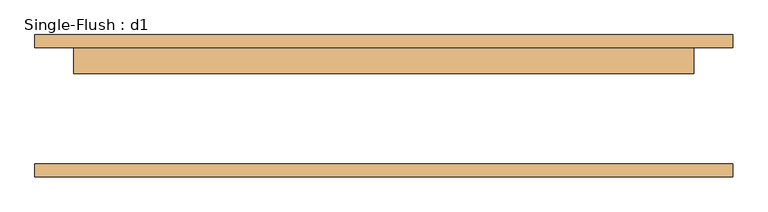
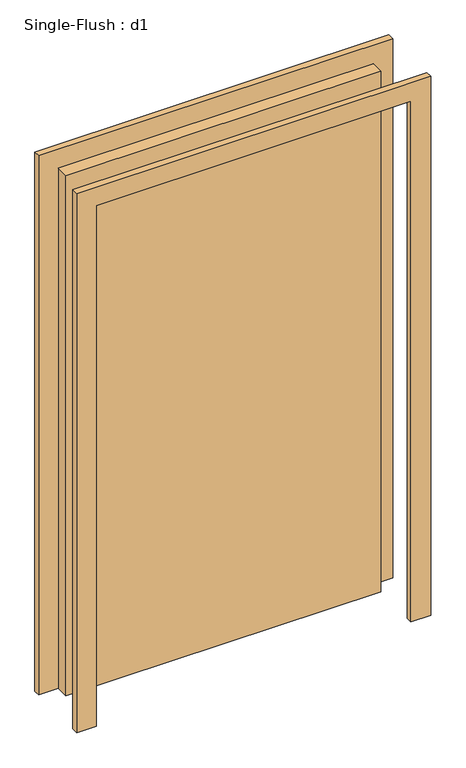
"""IFC4 building model written with IfcOpenShell, lengths in millimetres: door geometry, Single-Flush : d1."""

from ifc_helpers import new_model, si_unit, frame, origin, origin_with_axes, place, context, project, spatial, polyline, outline, extrude, source, transform, mapped, element, save


def single_flush_d1_2531c3a3(model_context):
    return source(origin(), model_context, "Body", "SweptSolid", [
        extrude(outline(polyline([(2209.8, -685.8), (0.0, -685.8), (0.0, -609.6), (2133.6, -609.6), (2133.6, 609.6), (0.0, 609.6), (0.0, 685.8), (2209.8, 685.8), (2209.8, -685.8)])), frame((0.0, 114.3, 0.0), z_axis=(0.0, 1.0, 0.0), x_axis=(0.0, 0.0, 1.0)), (0.0, 0.0, 1.0), 25.4),
        extrude(outline(polyline([(2209.8, 685.8), (2209.8, -685.8), (0.0, -685.8), (0.0, -609.6), (2133.6, -609.6), (2133.6, 609.6), (0.0, 609.6), (0.0, 685.8), (2209.8, 685.8)])), frame((0.0, -139.7, 0.0), z_axis=(0.0, 1.0, 0.0), x_axis=(0.0, 0.0, 1.0)), (0.0, 0.0, 1.0), 25.4),
        extrude(outline(polyline([(609.6, 63.5), (-609.6, 63.5), (-609.6, 114.3), (609.6, 114.3), (609.6, 63.5)])), origin_with_axes(), (0.0, 0.0, 1.0), 2133.6),
    ])


if __name__ == "__main__":
    model = new_model("IFC4")
    model_context = context("Model", 3, world=origin())
    ifc_project = project(units=[si_unit("LENGTHUNIT", "METRE", prefix="MILLI")], contexts=[model_context])
    site = spatial("IfcSite", under=ifc_project)
    building = spatial("IfcBuilding", under=site)
    placement = place(None, origin())
    single_flush_d1_shape = single_flush_d1_2531c3a3(model_context)
    element("IfcDoor", 1, ObjectType="Single-Flush : d1", at=placement, inside=building, context=model_context, shape_type="MappedRepresentation", body=[
        mapped(single_flush_d1_shape, transform((0.0, 0.0, 0.0), x_axis=(1.0, 0.0, 0.0), y_axis=(0.0, 1.0, 0.0), z_axis=(0.0, 0.0, 1.0))),
    ])
    save(model, "model.ifc")

# Revit data of these elements
# Type "Single-Flush : d1"
#   Type Mark = "8"
#   Construction Type Id = "MDOOR"
#   Assembly Code = "C1020"
#   Analytic Construction = "Metal"
#   Thickness = 0' - 2"
#   Heat Transfer Coefficient (U) = 0.651978 BTU/(h·ft²·°F)
#   Height = 7' - 0"
#   Trim Projection Ext = 0' - 1"
#   Trim Projection Int = 0' - 1"
#   Trim Width = 0' - 3"
#   Width = 4' - 0"
#   Define Thermal Properties by = 1
#   Door Material = Door - Panel
#   Frame Material = Door - Frame
#   Visual Light Transmittance = 0
#   Solar Heat Gain Coefficient = 0
#   Function = (empty or 0)
#   Wall Closure = (empty or 0)
# Element 1 (IfcDoor, "Single-Flush : d1")
#   Materials on its faces: "Door - Frame", "Door - Panel"
# Materials
#   "Door - Panel": class "Wood", colour RGB 210 159 95, transparency 0, Cost = 0
#   "Door - Frame": colour RGB 118 70 51, transparency 0, Cost = 0
